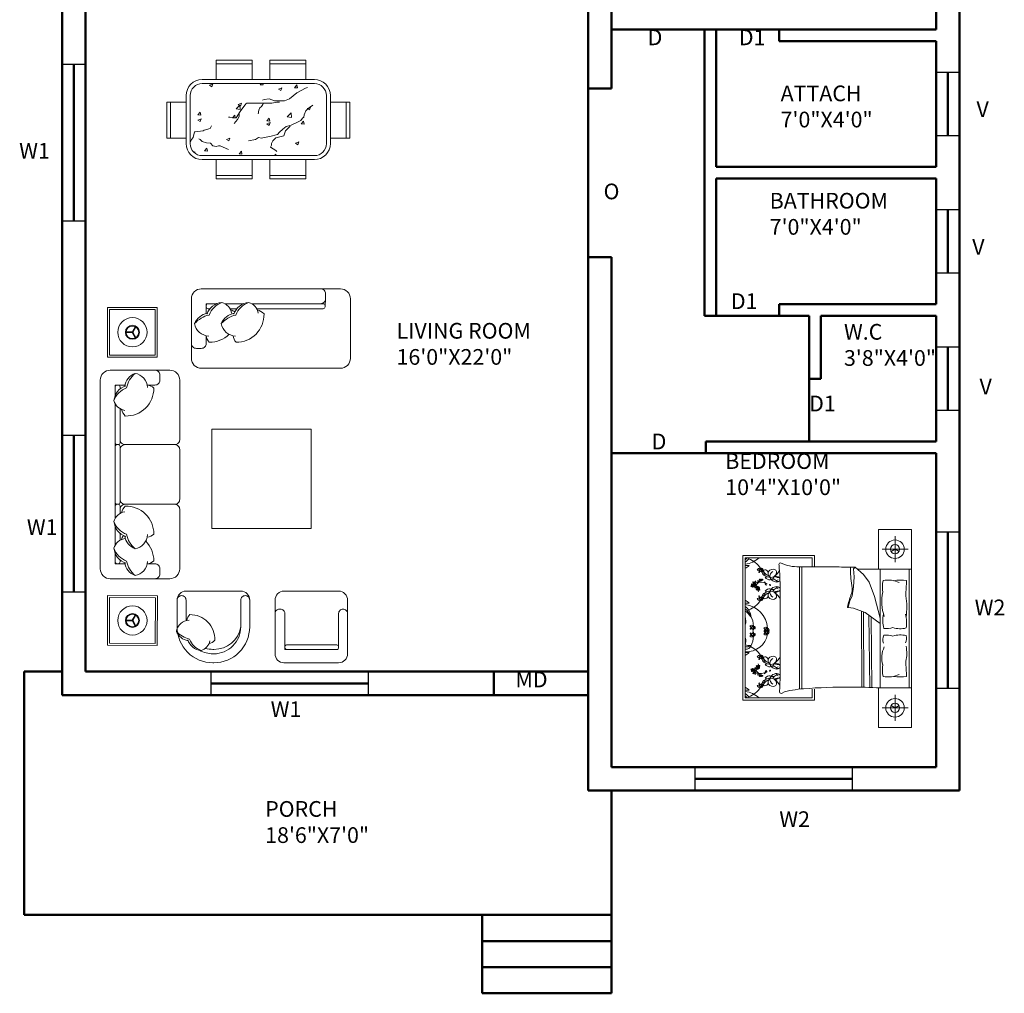
# Model space of a CAD drawing. Units: inches. Extents: x 18 to 447, y -515 to 49.
# Tile 1 of 2: x 71 to 447, y -515 to -143. Entities that reach past the tile are written whole.
import ezdxf

# ---------------------------------------------------------------- set-up
doc = ezdxf.new("R2010")
doc.units = ezdxf.units.IN
doc.header["$MEASUREMENT"] = 0
for name, color, linetype, lineweight in [('A-ANNO-TEXT', 7, 'Continuous', 25), ('A-AREA-IDEN', 3, 'Continuous', 25), ('A-FURN', 8, 'Continuous', 18), ('A-GLAZ', 4, 'Continuous', 25), ('A-WALL', 7, 'Continuous', 50)]:
    doc.layers.add(name, color=color, linetype=linetype, lineweight=lineweight)
doc.styles.get("Standard").update_dxf_attribs({"font": 'arial.ttf'})

# ---------------------------------------------------------------- blocks, each defined once
blk = doc.blocks.new('DAY BED1')
at = {"color": 0}
blk.add_line((0.3, 0.25), (0.225, 0.2549), dxfattribs=at)
blk.add_lwpolyline([(-0.3, 0, -0.414214), (-0.4, 0.1), (-0.4, 0.1, 0.317837), (-0.4, 0.1, -0.414214), (-0.4, 0.1), (-0.4, 0.1, 1.186185), (-0.4, 0.1, -0.414214), (-0.4, 0.1), (-0.4, 1.5, -0.414214), (-0.3, 1.6), (0.3, 1.6, -0.414214), (0.4, 1.5), (0.4, 0.1, -0.414214), (0.3, 0)], format="xyb", close=True, dxfattribs=at)
for points in [[(-0.0725, 1.45), (-0.15, 1.45, -0.414214), (-0.2, 1.5), (-0.2, 1.55, -0.414214), (-0.15, 1.6)], [(-0.0756, 1.4249, -0.356772), (0.0505, 1.5682, -0.249542), (0.1543, 1.4384, 9.61688)], [(0.0505, 1.5682, -0.14773), (0.1364, 1.422, -0.213343), (0.2624, 1.2931, -0.178662)], [(-0.0725, 1.4501, 0.165541), (-0.1386, 1.4192, 0.200231), (-0.0581, 1.2207, 0.121523)], [(0.1433, 1.4422, -0.306663), (0.2624, 1.2931, -0.30633), (0.1536, 1.1957, 0.872847)], [(0.25, 1.3448), (0.25, 1.45), (0.1517, 1.45, -0.414214)], [(0.2, 1.4118), (0.2, 1.43, -0.414214), (0.22, 1.45), (0.23, 1.45, -0.414214), (0.25, 1.43)], [(0.25, 1.43), (0.25, 1.3448, -0.414214)], [(-0.0756, 1.1556, -0.356772), (0.0505, 1.2988, -0.249542), (0.1543, 1.169, 9.61688)], [(0.0505, 1.2988, -0.14773), (0.1364, 1.1527, -0.213343), (0.2624, 1.0238, -0.178662)], [(0.1678, 1.1631, 0.071865), (0.1873, 1.205, -7.115464)], [(0.2, 1.1425), (0.2, 1.2113, -0.414214)], [(0.25, 1.2616), (0.25, 1.0755, -0.414214)], [(-0.0725, 1.1808, 0.165541), (-0.1386, 1.1498, 0.425989), (0.1479, 0.869, 0.121523), (0.1873, 0.9357, -7.115464)], [(0.1433, 1.1729, -0.306663), (0.2624, 1.0238, -0.30633), (0.1536, 0.9263, 0.872847)], [(0.25, 0.9923), (0.25, 0.2749, -0.414214), (0.23, 0.2549), (0.22, 0.2549, -0.414214), (0.2, 0.2749), (0.2, 0.9419, -0.414214)], [(0.25, 0.3775), (0.25, 0.3, 0.414214), (0.3, 0.25), (0.35, 0.25, 0.414214), (0.4, 0.3)]]:
    blk.add_lwpolyline(points, format="xyb", dxfattribs=at)
for points in [[(0.25, 1.0755), (0.25, 1.2616)], [(0.25, 0.3775), (0.25, 0.9923)]]:
    blk.add_lwpolyline(points, dxfattribs=at)
blk = doc.blocks.new('BED-DOUBLE')
for p, q in [((412.28, -42.96), (412.28, -33.06)), ((418.6, -30.43), (418.6, -106.23)), ((354.14, -40.44), (381.44, -40.44)), ((354.14, -95.69), (354.14, -40.44)), ((355.02, -41.31), (355.02, -94.82)), ((380.57, -41.31), (355.02, -41.31)), ((380.57, -44.72), (380.57, -41.31)), ((381.44, -40.44), (381.44, -44.72)), ((407.33, -38.01), (417.24, -38.01)), ((375.77, -91.48), (375.77, -44.72)), ((376.72, -91.41), (376.72, -44.72)), ((396.39, -45.53), (397.01, -44.91)), ((397.01, -44.91), (400.23, -47.67)), ((362.7, -48.78), (363.56, -48.62)), ((396.7, -48.6), (396.39, -45.53)), ((396.39, -52.43), (396.7, -48.6)), ((418.6, -45.59), (397.8, -45.59)), ((400.23, -47.67), (402.37, -50.59)), ((406.62, -45.59), (406.62, -91.07)), ((417.63, -91.07), (417.63, -45.59)), ((395.93, -55.81), (396.39, -52.43)), ((402.37, -50.59), (404.37, -56.12)), ((362.7, -54.08), (363.56, -54.25)), ((368.33, -83.72), (368.33, -52.94)), ((395.01, -57.81), (395.93, -55.81)), ((404.37, -56.12), (406.62, -64.38)), ((394.4, -60.26), (395.01, -57.81)), ((396.39, -60.57), (394.4, -60.26)), ((400.84, -62.26), (396.39, -60.57)), ((399.53, -90.8), (399.41, -61.72)), ((400.31, -90.8), (400.19, -62.01)), ((406.62, -66.41), (400.84, -62.26)), ((402.7, -90.83), (402.31, -63.31)), ((403.47, -90.86), (403.1, -63.88)), ((362.7, -82.05), (363.56, -81.88)), ((362.7, -87.35), (363.56, -87.51)), ((380.57, -94.82), (380.57, -91.47)), ((381.44, -91.49), (381.44, -95.69)), ((412.28, -93.7), (412.28, -103.6)), ((381.44, -95.69), (354.14, -95.69)), ((355.02, -94.82), (380.57, -94.82)), ((407.33, -98.65), (417.24, -98.65))]:
    blk.add_line(p, q)
for points in [[(405.97, -45.59), (405.97, -30.43), (418.6, -30.43)], [(412.28, -38.01), (410.75, -38.89)], [(412.28, -38.01), (413.82, -38.89)], [(418.6, -91.07), (405.97, -91.07), (405.97, -106.23), (418.6, -106.23)], [(412.28, -98.65), (410.75, -97.76)], [(412.28, -98.65), (413.82, -97.76)]]:
    blk.add_lwpolyline(points)
for points in [[(390.06, -44.75, 0.001242), (375.68, -44.72, -0.127202), (368.52, -43.2)], [(416.71, -49.94, 0.074897), (411.76, -50.04, -0.472817)], [(411.48, -67.97, 0.14099), (416.53, -68.13, 0.235245)], [(411.48, -71.21, -0.14099), (416.53, -71.06, -0.235245)], [(416.71, -86.71, -0.074897), (411.76, -86.62, 0.472817)], [(377.31, -91.39, 0.056112), (373.14, -91.94, 0.095341), (369.13, -93.01)]]:
    blk.add_lwpolyline(points, format="xyb")
for centre, radius in [((412.28, -38.01), 3.54), ((412.28, -38.01), 1.77), ((357.92, -51.9), 0.193), ((359.96, -53.16), 0.193), ((359.96, -82.97), 0.193), ((357.92, -84.23), 0.193), ((412.28, -98.65), 3.54), ((412.28, -98.65), 1.77)]:
    blk.add_circle(centre, radius)
for centre, radius, start, end in [((351.46, -37.17), 6.01, 306.3036, 316.4814), ((352.36, -38.91), 4.82, 303.4617, 330.1116), ((353.69, -33.94), 9.9, 277.745, 311.8856), ((353.48, -41.61), 4.02, 292.5547, 318.9546), ((355.64, -30.59), 13.69, 267.4081, 273.6519), ((352.71, -50.88), 9.9, 34.3865, 68.5908), ((368.56, -43.89), 0.699, 93.98, 207.3412), ((289.43, -52.04), 78.9, 359.3433, 5.6887), ((395.12, 24.59), 69.52, 265.8294, 271.553), ((423.85, -46.21), 28.61, 177.4519, 191.3392), ((360.64, -46.36), 1.1, 77.7115, 159.0387), ((360.05, -45.26), 0.827, 238.4633, 358.2869), ((362.76, -46.94), 2.5, 138.8402, 177.9352), ((360.38, -46.85), 0.123, 177.9352, 11.4834), ((360.44, -46.84), 0.0597, 11.4834, 127.9409), ((361.25, -46.01), 0.81, 117.6827, 223.7762), ((360.74, -46.49), 0.107, 223.7762, 159.7183), ((361.07, -46.09), 0.821, 2.9516, 103.728), ((367.63, -43.79), 6.92, 192.5173, 207.1824), ((359.96, -46.56), 1.56, 345.4653, 54.2343), ((362.32, -44.41), 1.69, 211.3827, 255.2969), ((362.98, -46.78), 1.42, 175.969, 254.3045), ((362.64, -47.05), 1.14, 350.264, 160.8688), ((361.41, -46.82), 0.697, 333.9755, 53.2681), ((361.1, -48.31), 1.51, 6.1662, 51.5825), ((365.15, -44.79), 3.58, 211.2614, 251.7045), ((364.86, -44.76), 4.07, 236.2883, 266.5076), ((364.34, -47.84), 1.88, 209.9085, 343.1337), ((365.56, -47.47), 1.81, 84.9449, 172.8857), ((365.96, -47.15), 2.2, 182.3591, 234.0401), ((366.25, -48.18), 1.76, 111.5819, 201.4221), ((364.8, -46.55), 2.28, 265.2933, 346.921), ((366.4, -51.29), 2.92, 122.7011, 126.3445), ((365.74, -46.94), 1.28, 354.4856, 91.0538), ((367.77, -45.7), 3.14, 238.8218, 279.1554), ((366.4, -51.29), 2.92, 55.785, 94.7304), ((362.99, -43.6), 5.74, 303.6671, 333.2997), ((367.49, -49.59), 0.913, 30.0293, 52.325), ((357.37, -52.19), 0.148, 142.4737, 265.053), ((357.56, -52.16), 0.319, 61.2196, 169.0403), ((357.4, -51.89), 0.449, 265.053, 338.3618), ((357.77, -51.51), 0.381, 157.4086, 261.4386), ((357.56, -51.49), 0.191, 58.0499, 135.6268), ((357.99, -52.51), 0.586, 113.4276, 137.6104), ((357.76, -51.61), 0.128, 172.906, 277.132), ((357.34, -51.85), 0.609, 14.7558, 58.0499), ((358.06, -52.25), 0.316, 139.7889, 227.6792), ((357.96, -52.36), 0.166, 227.6792, 350.3487), ((358.19, -51.69), 0.263, 36.1046, 181.4281), ((357.32, -52.24), 0.632, 353.0852, 15.7171), ((358.2, -50.65), 0.216, 124.3538, 214.3923), ((357.73, -52.32), 0.399, 350.3487, 43.6538), ((358.52, -50.69), 0.503, 190.3057, 287.1958), ((358.47, -51.91), 0.464, 198.7263, 262.5032), ((358.04, -51.48), 0.266, 270.0645, 331.1507), ((358.26, -51.54), 0.304, 221.8413, 265.7877), ((358.66, -50.51), 0.583, 176.9701, 248.2913), ((362.83, -47.43), 5.64, 212.6784, 216.3746), ((358.1, -52.12), 0.184, 1.1081, 91.8675), ((358.26, -51.66), 0.189, 263.7526, 41.7054), ((358.22, -52.17), 0.322, 11.5637, 86.365), ((358.47, -50.64), 0.223, 216.3746, 291.7548), ((360.44, -53.78), 3.15, 124.0033, 132.4917), ((358.45, -52.22), 0.149, 255.2356, 54.9248), ((357.21, -54.17), 3.36, 63.7819, 68.2913), ((359, -51.59), 0.535, 128.3208, 208.8162), ((359, -50.8), 0.503, 122.8155, 187.3992), ((359.1, -51.55), 0.639, 207.7043, 254.3516), ((358.61, -51.01), 0.168, 289.3605, 111.7548), ((358.74, -51.01), 0.168, 221.8703, 44.2646), ((359.5, -51.5), 0.88, 157.2305, 229.0635), ((359.22, -50.86), 0.583, 109.4799, 177.6828), ((359.21, -51.21), 0.518, 174.4544, 220.6188), ((358.68, -51.91), 0.88, 270.278, 342.111), ((359.27, -53.01), 0.622, 98.7227, 159.3375), ((356.26, -54.1), 3.78, 30.544, 49.818), ((358.91, -50.49), 0.216, 56.8636, 146.9021), ((359.02, -50.73), 0.223, 148.8844, 224.2646), ((358.34, -51.95), 0.622, 340.0041, 40.6188), ((363.66, -53.53), 5.64, 145.1882, 148.8844), ((360.44, -53.78), 3.15, 94.756, 119.2041), ((367.14, -58.31), 10.36, 132.2412, 142.1744), ((359.1, -51.89), 0.518, 278.7227, 324.8872), ((359, -52.31), 0.535, 290.5253, 358.5375), ((359.81, -52.77), 0.381, 157.4086, 261.4386), ((359.59, -52.76), 0.191, 58.0499, 135.6268), ((360.05, -52.15), 0.535, 182.8499, 266.1226), ((359.84, -51.78), 0.518, 231.7607, 277.9252), ((360.24, -51.68), 0.88, 214.5369, 286.3699), ((359.37, -53.11), 0.609, 14.7558, 58.0499), ((356.26, -54.1), 3.78, 23.0501, 23.8477), ((361.92, -50.06), 2.14, 178.3264, 187.1302), ((359.61, -50.36), 0.398, 11.3256, 64.4621), ((360.96, -49.79), 1.2, 190.2588, 210.656), ((360.15, -50.28), 0.364, 188.3432, 274.2869), ((360, -52.91), 0.622, 37.3105, 97.9252), ((360.47, -50.07), 0.635, 210.656, 242.6341), ((360.95, -49.53), 1.22, 218.2101, 226.3071), ((360.07, -52.05), 0.639, 265.0106, 311.658), ((360.05, -50.55), 0.154, 325.7657, 67.4417), ((355.26, -45.39), 7.2, 313.1541, 322.0459), ((360.6, -56.9), 6.28, 73.5842, 93.8277), ((360.55, -49.71), 0.148, 142.4737, 265.053), ((360.75, -49.68), 0.319, 127.7621, 169.0403), ((360.58, -49.41), 0.449, 265.053, 338.3618), ((361.17, -50.03), 0.586, 113.4276, 137.6104), ((361.1, -49.42), 0.193, 183.2768, 356.7232), ((361.25, -49.77), 0.316, 139.7889, 227.6792), ((361.15, -49.88), 0.166, 227.6792, 350.3487), ((360.5, -49.76), 0.632, 353.0852, 15.7171), ((360.92, -49.84), 0.399, 350.3487, 43.6538), ((361.66, -49.43), 0.464, 198.7263, 262.5032), ((361.29, -49.64), 0.184, 1.1081, 91.8675), ((361.63, -49.74), 0.149, 255.2356, 54.9248), ((361.4, -49.69), 0.322, 11.5637, 52.6358), ((364.47, -50.52), 2.14, 178.3264, 187.1302), ((362.16, -50.81), 0.398, 11.3256, 64.4621), ((363.51, -50.24), 1.2, 190.2588, 210.656), ((362.7, -50.73), 0.364, 188.3432, 274.2869), ((363.02, -50.53), 0.635, 210.656, 242.6341), ((363.5, -49.98), 1.22, 218.2101, 226.3071), ((362.6, -51), 0.154, 325.7657, 67.4417), ((363.04, -51.29), 0.364, 147.5332, 233.4768), ((363.37, -51.1), 0.635, 179.1859, 211.164), ((362.75, -51.24), 0.154, 354.3784, 96.0543), ((360.6, -56.9), 6.28, 63.0032, 69.8941), ((363.85, -50.81), 1.2, 211.164, 231.5612), ((364.06, -49.83), 2.14, 234.6898, 243.4936), ((364.07, -50.93), 1.22, 195.5129, 203.6099), ((362.71, -51.73), 0.398, 357.3579, 50.4944), ((364.42, -51.65), 0.146, 12.7051, 190.4384), ((364.51, -51.63), 0.238, 190.4384, 10.4136), ((365.13, -49.04), 0.47, 167.3041, 285.1471), ((366.95, -48.14), 2.42, 199.2822, 299.1751), ((366.95, -54.73), 2.42, 60.8249, 160.7178), ((365.66, -50.99), 1.55, 41.5653, 105.1471), ((366.51, -47.77), 2.18, 277.436, 299.9149), ((367.67, -49.21), 1.13, 221.5653, 293.8354), ((367.67, -53.66), 1.13, 66.1646, 138.4347), ((367.49, -49.59), 0.913, 314.4517, 333.558), ((367.49, -53.27), 0.913, 23.229, 45.5483), ((389.75, -53.05), 6.17, 336.2616, 11.3392), ((417.6, -52.65), 10.16, 165.1039, 191.0369), ((409.77, -59.6), 9.77, 65.1316, 101.7583), ((1138.04, -91.72), 722.54, 176.68521, 177.14978), ((358.96, -52.21), 0.639, 244.9899, 291.6373), ((359.4, -53.45), 0.148, 142.4737, 265.053), ((359.6, -53.42), 0.319, 61.2196, 169.0403), ((359.43, -53.16), 0.449, 265.053, 338.3618), ((360.02, -53.77), 0.586, 113.4276, 137.6104), ((359.79, -52.88), 0.128, 172.906, 277.132), ((360.1, -53.51), 0.316, 139.7889, 227.6792), ((360, -53.62), 0.166, 227.6792, 350.3487), ((360.23, -52.95), 0.263, 36.1046, 181.4281), ((359.35, -53.51), 0.632, 353.0852, 15.7171), ((356.26, -54.1), 3.78, 357.1071, 4.7585), ((359.77, -53.58), 0.399, 350.3487, 43.6538), ((360.07, -52.74), 0.266, 270.0645, 331.1507), ((360.3, -52.8), 0.304, 221.8413, 265.7877), ((360.51, -53.17), 0.464, 198.7263, 262.5032), ((360.14, -53.39), 0.184, 1.1081, 91.8675), ((360.38, -56.01), 0.123, 348.5166, 182.0648), ((362.76, -55.93), 2.5, 182.0648, 221.1598), ((360.3, -52.92), 0.189, 263.7526, 41.7054), ((360.26, -53.43), 0.322, 11.5637, 86.365), ((360.44, -56.03), 0.0597, 232.0591, 348.5166), ((361.25, -56.86), 0.81, 136.2238, 242.3173), ((360.49, -53.49), 0.149, 255.2356, 54.9248), ((360.78, -56.38), 0.0645, 200.2667, 136.2271), ((359.96, -56.3), 1.56, 305.7657, 14.5347), ((367.63, -59.08), 6.92, 152.8176, 167.4827), ((362.98, -56.09), 1.42, 105.6955, 184.031), ((362.64, -55.81), 1.14, 199.1312, 9.736), ((361.41, -56.05), 0.697, 306.7319, 26.0245), ((361.1, -54.56), 1.51, 308.4175, 353.8338), ((365.15, -58.07), 3.58, 108.2955, 148.7386), ((364.86, -58.1), 4.07, 93.4924, 123.7117), ((364.34, -55.02), 1.88, 16.8663, 150.0915), ((365.96, -55.71), 2.2, 125.9599, 177.6409), ((365.56, -55.4), 1.81, 187.1143, 275.0551), ((366.25, -54.69), 1.76, 158.5779, 248.4181), ((364.8, -56.31), 2.28, 13.079, 94.7067), ((365.13, -53.83), 0.47, 74.8529, 192.6959), ((366.4, -51.58), 2.92, 233.6555, 237.2989), ((365.66, -51.87), 1.55, 254.8529, 318.4347), ((365.74, -55.92), 1.28, 268.9462, 5.5144), ((367.77, -57.16), 3.14, 79.7133, 121.1782), ((366.4, -51.58), 2.92, 265.2696, 304.215), ((362.99, -59.26), 5.74, 21.4941, 56.3329), ((366.51, -55.09), 2.18, 60.0851, 82.564), ((367.49, -53.27), 0.913, 307.675, 336.7144), ((423.04, -65.53), 29.39, 160.1194, 169.3383), ((424.82, -57.99), 17.62, 168.0397, 199.2615), ((389.28, -60.33), 27.49, 352.2196, 9.497), ((353.48, -61.25), 4.02, 41.0454, 67.4453), ((355.64, -72.28), 13.69, 86.3481, 92.5919), ((353.69, -68.92), 9.9, 4.4623, 82.255), ((352.36, -63.95), 4.82, 1.272, 56.5383), ((352.71, -51.98), 9.9, 291.4092, 325.6135), ((360.05, -57.6), 0.827, 1.7131, 121.5367), ((360.64, -56.5), 1.1, 200.9613, 282.2885), ((361.07, -56.78), 0.821, 256.272, 357.0484), ((362.32, -58.45), 1.69, 104.7031, 148.6173), ((394.34, -60.09), 0.183, 178.8623, 289.7536), ((351.46, -65.69), 6.01, 17.8504, 53.6964), ((349.77, -68.85), 8.94, 34.0123, 54.053), ((349.81, -65.39), 5.44, 343.5431, 17.0202), ((348.38, -68.16), 9.9, 4.4623, 27.4146), ((420.97, -65.13), 13.37, 169.8617, 193.6238), ((403.18, -66.14), 13.51, 351.5249, 13.96), ((347.01, -67.55), 8.05, 4.3787, 5.6357), ((341.5, -71.79), 14.38, 19.7217, 19.9028), ((357.51, -68.2), 1.1, 47.7873, 129.1145), ((357.55, -66.96), 0.827, 208.5391, 328.3627), ((359.06, -69.76), 2.5, 108.9159, 148.011), ((358.22, -68.2), 0.81, 87.7585, 193.852), ((364.86, -69.46), 6.92, 162.593, 177.2582), ((356.83, -68.03), 1.56, 315.5411, 24.3101), ((359.94, -67.35), 1.69, 181.4585, 225.3727), ((358.02, -68.18), 0.821, 333.0274, 73.8037), ((355.97, -69.42), 7.66, 262.8636, 351.8197), ((357.55, -71.7), 0.827, 31.6373, 151.4609), ((357.51, -70.45), 1.1, 230.8855, 312.2127), ((357.04, -68.5), 0.123, 148.011, 341.5592), ((357.04, -70.16), 0.123, 18.4408, 211.989), ((359.06, -68.9), 2.5, 211.989, 251.0841), ((357.1, -68.52), 0.0597, 341.5592, 98.0167), ((357.1, -70.14), 0.0597, 261.9833, 18.4408), ((348.38, -70.5), 9.9, 332.5854, 355.5377), ((358.22, -70.46), 0.81, 166.148, 272.2415), ((357.54, -68.37), 0.107, 193.852, 129.9245), ((357.58, -70.28), 0.0645, 230.1909, 166.0209), ((364.86, -69.19), 6.92, 182.7418, 197.407), ((356.83, -70.62), 1.56, 335.6899, 44.4589), ((359.94, -71.31), 1.69, 134.6273, 178.5415), ((358.02, -70.48), 0.821, 286.1963, 26.9726), ((362.82, -68.96), 1.1, 47.7873, 129.1145), ((362.85, -67.71), 0.827, 208.5391, 328.3627), ((362.85, -70.94), 0.827, 31.6373, 151.4609), ((362.82, -69.69), 1.1, 230.8855, 312.2127), ((362.35, -69.26), 0.123, 148.011, 341.5592), ((362.35, -69.4), 0.123, 18.4408, 211.989), ((364.36, -70.52), 2.5, 108.9159, 148.011), ((364.36, -68.14), 2.5, 211.989, 251.0841), ((362.41, -69.28), 0.0597, 341.5592, 98.0167), ((362.41, -69.38), 0.0597, 261.9833, 18.4408), ((363.52, -68.96), 0.81, 87.7585, 193.852), ((363.52, -69.7), 0.81, 166.148, 272.2415), ((362.84, -69.13), 0.107, 193.852, 129.9245), ((362.88, -69.52), 0.0645, 230.1909, 166.0209), ((362.13, -68.79), 1.56, 315.5411, 24.3101), ((370.16, -70.22), 6.92, 162.593, 177.2582), ((362.13, -69.86), 1.56, 335.6899, 44.4589), ((370.16, -68.44), 6.92, 182.7418, 197.407), ((363.32, -68.94), 0.821, 333.0274, 73.8037), ((365.24, -68.11), 1.69, 181.4585, 225.3727), ((363.32, -69.72), 0.821, 286.1963, 26.9726), ((365.24, -70.55), 1.69, 134.6273, 178.5415), ((411.62, -72.61), 4.02, 155.0183, 198.5407), ((408.95, -59.04), 9.29, 264.0129, 285.8293), ((408.95, -80.15), 9.29, 74.1707, 95.9871), ((412.93, -72.1), 3.75, 333.3437, 16.1026), ((349.81, -73.26), 5.44, 342.9798, 16.4569), ((347.01, -71.11), 8.05, 354.3643, 355.6213), ((341.5, -66.87), 14.38, 340.0972, 340.2783), ((356.67, -70.41), 4.43, 248.117, 276.6195), ((355.44, -74.47), 1.78, 256.3898, 349.0739), ((355.68, -73.14), 2.25, 252.8609, 311.9049), ((352.71, -84.14), 9.9, 34.3865, 68.5908), ((403.45, -77.72), 13.32, 346.3427, 11.1841), ((355.64, -63.85), 13.69, 267.4081, 273.6519), ((353.48, -74.88), 4.02, 292.5547, 318.9546), ((360.64, -79.63), 1.1, 77.7115, 159.0387), ((360.05, -78.53), 0.827, 238.4633, 358.2869), ((362.76, -80.2), 2.5, 138.8402, 177.9352), ((361.25, -79.27), 0.81, 117.6827, 223.7762), ((361.07, -79.35), 0.821, 2.9516, 103.728), ((362.32, -77.67), 1.69, 211.3827, 255.2969), ((359.96, -79.82), 1.56, 345.4653, 54.2343), ((367.63, -77.05), 6.92, 192.5173, 207.1824), ((365.56, -80.73), 1.81, 84.9449, 172.8857), ((365.74, -80.21), 1.28, 354.4856, 91.0538), ((362.99, -76.87), 5.74, 303.6671, 338.5059), ((416.85, -79.63), 9.65, 153.8761, 196.1746), ((359.4, -82.67), 0.148, 94.947, 217.5263), ((359.6, -82.7), 0.319, 190.9597, 298.7804), ((359.43, -82.97), 0.449, 21.6382, 94.947), ((360.02, -82.36), 0.586, 222.3896, 246.5724), ((360.1, -82.62), 0.316, 132.3208, 220.2111), ((360, -82.51), 0.166, 9.6513, 132.3208), ((359.35, -82.62), 0.632, 344.2829, 6.9148), ((356.26, -82.03), 3.78, 355.2415, 2.8929), ((359.77, -82.55), 0.399, 316.3462, 9.6513), ((360.51, -82.96), 0.464, 97.4968, 161.2737), ((360.14, -82.74), 0.184, 268.1325, 358.8919), ((360.38, -80.12), 0.123, 177.9352, 11.4834), ((360.26, -82.7), 0.322, 273.635, 348.4363), ((360.44, -80.1), 0.0597, 11.4834, 127.9409), ((360.49, -82.64), 0.149, 305.0752, 104.7644), ((360.74, -79.76), 0.107, 223.7762, 159.7183), ((362.98, -80.04), 1.42, 175.969, 254.3045), ((362.64, -80.32), 1.14, 350.264, 160.8688), ((361.41, -80.08), 0.697, 333.9755, 53.2681), ((361.1, -81.57), 1.51, 6.1662, 51.5825), ((365.15, -78.06), 3.58, 211.2614, 251.7045), ((364.86, -78.03), 4.07, 236.2883, 266.5076), ((364.34, -81.11), 1.88, 209.9085, 343.1337), ((365.96, -80.42), 2.2, 182.3591, 234.0401), ((366.25, -81.44), 1.76, 111.5819, 201.4221), ((364.8, -79.81), 2.28, 265.2933, 346.921), ((365.13, -82.3), 0.47, 167.3041, 285.1471), ((366.4, -84.55), 2.92, 122.7011, 126.3445), ((366.95, -81.4), 2.42, 199.2822, 299.1751), ((365.66, -84.26), 1.55, 41.5653, 105.1471), ((367.77, -78.97), 3.14, 238.8218, 280.2867), ((366.4, -84.55), 2.92, 55.785, 94.7304), ((367.49, -82.86), 0.913, 23.2856, 52.325), ((417.6, -84.01), 10.16, 168.9631, 194.8961), ((1138.04, -44.94), 722.54, 182.85022, 183.31479), ((357.37, -83.94), 0.148, 94.947, 217.5263), ((357.56, -83.97), 0.319, 190.9597, 298.7804), ((357.4, -84.24), 0.449, 21.6382, 94.947), ((357.77, -84.62), 0.381, 98.5614, 202.5914), ((357.56, -84.64), 0.191, 224.3732, 301.9501), ((357.99, -83.62), 0.586, 222.3896, 246.5724), ((357.76, -84.52), 0.128, 82.868, 187.094), ((357.34, -84.28), 0.609, 301.9501, 345.2442), ((358.06, -83.88), 0.316, 132.3208, 220.2111), ((357.96, -83.77), 0.166, 9.6513, 132.3208), ((357.32, -83.88), 0.632, 344.2829, 6.9148), ((358.19, -84.44), 0.263, 178.5719, 323.8954), ((358.2, -85.47), 0.216, 145.6077, 235.6462), ((357.73, -83.81), 0.399, 316.3462, 9.6513), ((358.47, -84.22), 0.464, 97.4968, 161.2737), ((358.52, -85.44), 0.503, 72.8042, 169.6943), ((358.26, -84.59), 0.304, 94.2123, 138.1587), ((358.04, -84.65), 0.266, 28.8493, 89.9355), ((358.66, -85.62), 0.583, 111.7087, 183.0299), ((362.83, -88.7), 5.64, 143.6254, 147.3216), ((358.1, -84), 0.184, 268.1325, 358.8919), ((358.22, -83.96), 0.322, 273.635, 348.4363), ((358.26, -84.47), 0.189, 318.2946, 96.2474), ((358.47, -85.49), 0.223, 68.2452, 143.6254), ((360.44, -82.35), 3.15, 227.5083, 235.9967), ((358.45, -83.91), 0.149, 305.0752, 104.7644), ((357.21, -81.96), 3.36, 291.7087, 296.2181), ((359, -84.54), 0.535, 151.1838, 231.6792), ((359, -85.33), 0.503, 172.6008, 237.1845), ((359.1, -84.58), 0.639, 105.6484, 152.2957), ((358.61, -85.12), 0.168, 248.2452, 70.6395), ((358.74, -85.12), 0.168, 315.7354, 138.1297), ((359.5, -84.63), 0.88, 130.9365, 202.7695), ((359.22, -85.26), 0.583, 182.3172, 250.5201), ((358.96, -83.92), 0.639, 68.3627, 115.0101), ((358.68, -84.22), 0.88, 17.889, 89.722), ((359.27, -83.12), 0.622, 200.6625, 261.2773), ((359.21, -84.92), 0.518, 139.3812, 185.5456), ((356.26, -82.03), 3.78, 310.182, 329.456), ((358.91, -85.63), 0.216, 213.0979, 303.1364), ((359.02, -85.39), 0.223, 135.7354, 211.1156), ((358.34, -84.18), 0.622, 319.3812, 19.9959), ((363.66, -82.6), 5.64, 211.1156, 214.8118), ((360.44, -82.35), 3.15, 240.7959, 265.244), ((367.14, -77.82), 10.36, 217.8256, 227.7588), ((359.1, -84.24), 0.518, 35.1128, 81.2773), ((359, -83.82), 0.535, 1.4625, 69.4747), ((359.81, -83.36), 0.381, 98.5614, 202.5914), ((359.59, -83.37), 0.191, 224.3732, 301.9501), ((360.05, -83.98), 0.535, 93.8774, 177.1501), ((360.24, -84.44), 0.88, 73.6301, 145.4631), ((359.84, -84.35), 0.518, 82.0748, 128.2393), ((359.79, -83.25), 0.128, 82.868, 187.094), ((359.37, -83.02), 0.609, 301.9501, 345.2442), ((356.26, -82.03), 3.78, 336.1523, 336.9499), ((360.96, -86.34), 1.2, 149.344, 169.7412), ((361.92, -86.07), 2.14, 172.8698, 181.6736), ((359.61, -85.77), 0.398, 295.5379, 348.6744), ((360.15, -85.85), 0.364, 85.7131, 171.6568), ((360, -83.22), 0.622, 262.0748, 322.6895), ((360.47, -86.05), 0.635, 117.3659, 149.344), ((360.23, -83.18), 0.263, 178.5719, 323.8954), ((360.95, -86.6), 1.22, 133.6929, 141.7899), ((360.07, -84.08), 0.639, 48.342, 94.9894), ((360.3, -83.32), 0.304, 94.2123, 138.1587), ((360.07, -83.39), 0.266, 28.8493, 89.9355), ((360.05, -85.58), 0.154, 292.5583, 34.2343), ((360.6, -79.23), 6.28, 266.1723, 286.4158), ((355.26, -90.74), 7.2, 37.9541, 46.8459), ((360.3, -83.21), 0.189, 318.2946, 96.2474), ((360.55, -86.42), 0.148, 94.947, 217.5263), ((360.75, -86.45), 0.319, 190.9597, 232.2379), ((360.58, -86.72), 0.449, 21.6382, 94.947), ((361.17, -86.1), 0.586, 222.3896, 246.5724), ((361.1, -86.71), 0.193, 3.2768, 176.7232), ((361.25, -86.36), 0.316, 132.3208, 220.2111), ((361.15, -86.25), 0.166, 9.6513, 132.3208), ((360.5, -86.36), 0.632, 344.2829, 6.9148), ((360.92, -86.29), 0.399, 316.3462, 9.6513), ((361.66, -86.7), 0.464, 97.4968, 161.2737), ((361.29, -86.48), 0.184, 268.1325, 358.8919), ((361.63, -86.38), 0.149, 305.0752, 104.7644), ((361.4, -86.44), 0.322, 307.3642, 348.4363), ((363.51, -85.89), 1.2, 149.344, 169.7412), ((364.47, -85.61), 2.14, 172.8698, 181.6736), ((362.16, -85.32), 0.398, 295.5379, 348.6744), ((362.7, -85.4), 0.364, 85.7131, 171.6568), ((363.02, -85.6), 0.635, 117.3659, 149.344), ((363.5, -86.15), 1.22, 133.6929, 141.7899), ((362.6, -85.13), 0.154, 292.5583, 34.2343), ((363.04, -84.84), 0.364, 126.5232, 212.4668), ((364.34, -88.29), 1.88, 16.8663, 150.0915), ((363.37, -85.03), 0.635, 148.836, 180.8141), ((362.75, -84.88), 0.154, 263.9457, 5.6216), ((360.6, -79.23), 6.28, 290.1059, 296.9968), ((363.85, -85.32), 1.2, 128.4388, 148.836), ((364.06, -86.3), 2.14, 116.5064, 125.3102), ((364.07, -85.2), 1.22, 156.3901, 164.4871), ((362.71, -84.4), 0.398, 309.5056, 2.6421), ((364.51, -84.5), 0.238, 349.5864, 169.5616), ((364.42, -84.48), 0.146, 169.5616, 347.2949), ((366.95, -87.99), 2.42, 60.8249, 160.7178), ((365.66, -85.14), 1.55, 254.8529, 318.4347), ((366.51, -81.04), 2.18, 277.436, 299.9149), ((366.51, -88.36), 2.18, 60.0851, 82.564), ((367.67, -82.47), 1.13, 221.5653, 293.8354), ((367.67, -86.92), 1.13, 66.1646, 138.4347), ((294.61, -86.04), 73.76, 355.2402, 1.8035), ((367.49, -82.86), 0.913, 314.4517, 336.7144), ((367.49, -86.54), 0.913, 16.6343, 45.5483), ((409.77, -77.06), 9.77, 258.2417, 294.8684), ((360.05, -90.87), 0.827, 1.7131, 121.5367), ((360.64, -89.77), 1.1, 200.9613, 282.2885), ((360.38, -89.28), 0.123, 348.5166, 182.0648), ((362.76, -89.19), 2.5, 182.0648, 221.1598), ((360.44, -89.29), 0.0597, 232.0591, 348.5166), ((361.25, -90.12), 0.81, 136.2238, 242.3173), ((360.78, -89.65), 0.0645, 200.2667, 136.2271), ((367.63, -92.34), 6.92, 152.8176, 167.4827), ((359.96, -89.57), 1.56, 305.7657, 14.5347), ((362.32, -91.72), 1.69, 104.7031, 148.6173), ((361.07, -90.04), 0.821, 256.272, 357.0484), ((362.98, -89.35), 1.42, 105.6955, 184.031), ((362.64, -89.08), 1.14, 199.1312, 9.736), ((361.41, -89.31), 0.697, 306.7319, 26.0245), ((361.1, -87.82), 1.51, 308.4175, 353.8338), ((365.15, -91.34), 3.58, 108.2955, 148.7386), ((364.86, -91.37), 4.07, 93.4924, 123.7117), ((365.96, -88.98), 2.2, 125.9599, 177.6409), ((365.56, -88.66), 1.81, 187.1143, 275.0551), ((366.25, -87.95), 1.76, 158.5779, 248.4181), ((364.8, -89.58), 2.28, 13.079, 94.7067), ((365.13, -87.09), 0.47, 74.8529, 192.6959), ((366.4, -84.84), 2.92, 233.6555, 237.2989), ((365.74, -89.19), 1.28, 268.9462, 5.5144), ((367.77, -90.43), 3.14, 79.249, 121.1782), ((366.4, -84.84), 2.92, 265.2696, 304.215), ((362.99, -92.53), 5.74, 23.6453, 56.3329), ((367.49, -86.54), 0.913, 307.675, 342.5814), ((353.48, -94.52), 4.02, 41.0454, 67.4453), ((355.64, -105.54), 13.69, 86.3481, 92.5919), ((353.69, -102.18), 9.9, 48.1144, 82.255), ((352.36, -97.22), 4.82, 29.8884, 56.5383), ((352.71, -85.25), 9.9, 291.4092, 325.6135), ((368.74, -92.43), 0.691, 156.5219, 303.8264), ((392.41, -268.41), 177.66, 89.1145, 94.8735), ((397.36, -226.95), 136.19, 86.1, 90.9282), ((351.46, -98.95), 6.01, 43.5186, 53.6964)]:
    blk.add_arc(centre, radius, start, end)
blk = doc.blocks.new('SIDE-TABLE-LAMP')
for p, q in [((114.05, -262.6), (111.38, -262.6)), ((114.05, -262.84), (111.38, -262.84)), ((113.95, -262.66), (115.29, -260.34)), ((113.95, -262.78), (115.29, -265.1)), ((114.16, -262.78), (115.5, -260.46)), ((114.16, -262.66), (115.5, -264.98))]:
    blk.add_line(p, q)
at = {"ltscale": 0.03}
blk.add_lwpolyline([(123.55, -253.23), (123.55, -272.22), (104.56, -272.22), (104.56, -253.23)], close=True, dxfattribs=at)
blk.add_lwpolyline([(122.79, -271.46), (122.79, -253.99), (105.32, -253.99), (105.32, -271.46)], close=True)
for radius in [5.6, 2.68, 2.4]:
    blk.add_circle((114.05, -262.72), radius)
blk = doc.blocks.new('CHAIR-DINING')
for p, q in [((7.38, 13.77), (0, 13.77)), ((7.38, 0), (7.38, 13.77)), ((0, 0), (7.38, 0))]:
    blk.add_line(p, q)
blk = doc.blocks.new('WIN-W')
for p, q in [((0, 9), (60, 9)), ((0, 0), (0, 9)), ((60, 9), (60, 0)), ((60, 0), (0, 0))]:
    blk.add_line(p, q)
blk = doc.blocks.new('WIN-V')
for p, q in [((0, 24), (0, 0)), ((9, 24), (0, 24)), ((9, 0), (9, 24)), ((0, 0), (9, 0))]:
    blk.add_line(p, q)

msp = doc.modelspace()

# ---------------------------------------------------------------- linework, layer by layer
at = {"layer": 'A-FURN'}
for p, q in [((159.8, -160.07), (146.02, -160.07)), ((180.31, -160.07), (166.53, -160.07)), ((183.58, -166.1), (140.73, -166.1)), ((140.73, -167.63), (183.58, -167.63)), ((143.51, -168.24), (144.8, -167.75)), ((143.51, -168.24), (144.42, -168.86)), ((144.42, -168.86), (144.8, -167.75)), ((162.87, -168.05), (163.22, -167.63)), ((162.87, -168.05), (163.97, -168.15)), ((163.97, -168.15), (163.87, -167.63)), ((169.9, -169.71), (171.19, -169.22)), ((170.82, -170.33), (171.19, -169.22)), ((176.04, -169.2), (176.93, -168.15)), ((176.04, -169.2), (177.14, -169.3)), ((177.14, -169.3), (176.93, -168.15)), ((181.02, -169.11), (180.19, -169.44)), ((134.61, -172.22), (134.61, -190.59)), ((136.14, -190.59), (136.14, -172.22)), ((169.9, -169.71), (170.82, -170.33)), ((176.86, -171.11), (174.03, -173.43)), ((180.19, -169.44), (176.86, -171.11)), ((188.17, -172.22), (188.17, -190.59)), ((189.7, -190.59), (189.7, -172.22)), ((128.58, -188.48), (128.58, -174.7)), ((153.65, -177.31), (155.08, -175.82)), ((154.47, -175.64), (155.76, -175.14)), ((154.47, -175.64), (155.39, -176.25)), ((155.28, -177.56), (155.08, -175.82)), ((157.39, -175.43), (155.22, -178.25)), ((155.39, -176.25), (155.76, -175.14)), ((157.72, -175.1), (157.39, -175.43)), ((167.37, -175.1), (157.72, -175.1)), ((163.38, -176.42), (162.72, -176.92)), ((163.88, -175.59), (163.38, -176.42)), ((164.38, -173.77), (163.71, -173.93)), ((164.21, -175.09), (163.88, -175.59)), ((166.37, -173.43), (164.38, -173.77)), ((168.37, -174.26), (166.37, -173.43)), ((169.2, -174.76), (167.37, -175.1)), ((172.2, -174.26), (168.37, -174.26)), ((170.2, -174.76), (169.2, -174.76)), ((174.03, -173.43), (172.2, -174.26)), ((181.68, -176.76), (180.35, -178.09)), ((180.86, -177.11), (182.15, -176.61)), ((183.02, -175.93), (181.68, -176.76)), ((181.78, -177.72), (182.15, -176.61)), ((195.73, -174.7), (195.73, -188.48)), ((139.07, -179.56), (139.96, -178.51)), ((139.07, -179.56), (140.17, -179.66)), ((140.17, -179.66), (139.96, -178.51)), ((151.23, -180.42), (150.73, -180.42)), ((153.73, -180.75), (151.23, -180.42)), ((152.24, -180.71), (153.13, -179.66)), ((153.34, -180.81), (153.13, -179.66)), ((153.65, -177.31), (155.28, -177.56)), ((155.22, -178.25), (153.73, -180.75)), ((154.89, -180.25), (154.23, -181.41)), ((154.89, -178.75), (154.89, -180.25)), ((162.22, -178.75), (162.05, -179.25)), ((162.38, -177.75), (162.22, -178.41)), ((162.22, -178.41), (162.22, -178.75)), ((162.72, -176.92), (162.38, -177.75)), ((173.25, -180.35), (174.68, -178.85)), ((173.25, -180.35), (174.88, -180.6)), ((174.88, -180.6), (174.68, -178.86)), ((179.52, -180.42), (179.02, -180.91)), ((179.69, -179.58), (179.52, -180.42)), ((180.35, -178.09), (179.69, -179.58)), ((180.86, -177.11), (181.78, -177.72)), ((139.04, -181.56), (140.33, -181.07)), ((139.04, -181.56), (139.95, -182.18)), ((139.95, -182.18), (140.33, -181.07)), ((143.74, -184.74), (144.24, -183.74)), ((152.24, -180.71), (153.34, -180.81)), ((153.56, -182.08), (152.89, -182.91)), ((154.23, -181.41), (153.56, -182.08)), ((165.42, -181.87), (166.3, -180.81)), ((165.42, -181.87), (166.51, -181.96)), ((165.43, -183.03), (166.72, -182.54)), ((165.43, -183.03), (166.35, -183.65)), ((166.51, -181.96), (166.3, -180.81)), ((166.35, -183.65), (166.72, -182.54)), ((172.86, -184.07), (171.53, -185.07)), ((174.69, -183.57), (172.86, -184.07)), ((174.36, -183.91), (173.7, -184.57)), ((177.19, -182.41), (174.69, -183.57)), ((178.36, -181.74), (177.19, -182.41)), ((179.02, -180.91), (178.36, -181.74)), ((178.59, -183.02), (179.47, -181.96)), ((178.59, -183.02), (179.69, -183.11)), ((179.69, -183.12), (179.47, -181.96)), ((137.25, -188.23), (137.75, -186.07)), ((137.75, -186.07), (138.08, -186.07)), ((138.08, -186.07), (141.08, -185.73)), ((141.08, -185.73), (141.41, -185.4)), ((141.41, -185.4), (143.74, -184.74)), ((166.54, -187.89), (164.38, -188.23)), ((169.54, -187.06), (166.54, -187.89)), ((171.87, -187.56), (168.87, -188.39)), ((170.2, -186.23), (169.54, -187.06)), ((171.53, -185.07), (170.2, -186.23)), ((172.03, -187.23), (171.87, -187.56)), ((172.53, -185.73), (172.03, -187.23)), ((173.7, -184.57), (172.53, -185.73)), ((136.25, -189.89), (136.59, -189.06)), ((136.59, -189.06), (137.25, -188.23)), ((139.92, -189.05), (139.42, -188.72)), ((140.75, -189.72), (139.92, -189.05)), ((142.41, -190.22), (140.75, -189.72)), ((143.91, -190.38), (142.41, -190.22)), ((144.74, -191.38), (143.91, -190.38)), ((146.07, -191.71), (144.74, -191.38)), ((146.91, -191.38), (146.07, -191.71)), ((147.57, -191.38), (146.91, -191.38)), ((150.73, -192.88), (147.57, -191.38)), ((150, -188.95), (151.29, -188.46)), ((150, -188.95), (150.92, -189.57)), ((150.92, -189.57), (151.29, -188.46)), ((161.05, -189.06), (158.39, -189.56)), ((162.21, -188.23), (161.05, -189.06)), ((163.38, -188.56), (162.21, -188.23)), ((164.38, -188.23), (163.38, -188.56)), ((167.21, -191.22), (166.87, -191.88)), ((166.87, -191.88), (168.87, -193.21)), ((167.71, -189.56), (167.21, -190.55)), ((167.21, -190.55), (167.21, -191.22)), ((168.87, -188.39), (167.71, -189.56)), ((176.4, -190.43), (177.68, -189.93)), ((176.4, -190.43), (177.31, -191.04)), ((177.31, -191.04), (177.68, -189.93)), ((137.64, -193.99), (137.91, -193.71)), ((137.98, -194.26), (137.91, -193.71)), ((183.58, -195.18), (140.73, -195.18)), ((141.62, -193.38), (142.5, -192.32)), ((141.62, -193.38), (142.72, -193.47)), ((142.72, -193.47), (142.5, -192.32)), ((154.79, -194.53), (155.68, -193.47)), ((154.79, -194.53), (155.89, -194.62)), ((155.89, -194.62), (155.68, -193.47)), ((168.39, -195.18), (168.85, -194.63)), ((168.95, -195.18), (168.85, -194.63)), ((168.87, -193.21), (169.2, -193.55)), ((140.73, -196.71), (183.58, -196.71)), ((159.8, -202.74), (146.02, -202.74)), ((180.31, -202.74), (166.53, -202.74))]:
    msp.add_line(p, q, dxfattribs=at)
at = {"layer": 'A-FURN', "ltscale": 0.03}
for points in [[(128.35, -277.2, -0.414214), (132.14, -281), (132.14, -303.79, -0.414214), (130.24, -305.68, -0.414214), (132.14, -307.58), (132.14, -326.57, -0.414214), (130.24, -328.47, -0.414214), (132.14, -330.37), (132.14, -353.15, -0.414214), (128.35, -356.95), (105.56, -356.95, -0.414214), (101.76, -353.15), (101.76, -281, -0.414214), (105.56, -277.2)], [(192.86, -389.08), (192.86, -389.08, 0.414214), (196.28, -385.65), (196.28, -365.11, 0.414214), (192.86, -361.69), (192.86, -361.69), (171.97, -361.69, 0.414214), (168.55, -365.11), (168.55, -385.65, 0.414214), (171.97, -389.08)]]:
    msp.add_lwpolyline(points, format="xyb", close=True, dxfattribs=at)
at = {"layer": 'A-FURN'}
for points in [[(115.04, -278.41, 0.14773), (111.77, -283.96, 0.213343), (106.99, -288.86, 0.178662)], [(119.82, -283.85, 0.356772), (115.04, -278.41, 0.249542), (111.09, -283.34, -9.61688)], [(122.65, -277.2, -0.414214), (124.55, -279.1), (124.55, -281, -0.414214), (122.65, -282.9), (119.71, -282.9)], [(111.51, -283.19, 0.306663), (106.99, -288.86, 0.30633), (111.12, -292.56, -0.872847)], [(109.36, -284.35), (109.36, -283.66, 0.414214), (108.6, -282.9), (108.22, -282.9, 0.414214), (107.46, -283.66)], [(107.46, -283.66), (107.46, -286.89, 0.414214)], [(119.71, -282.9, -0.165541), (122.22, -284.07, -0.425989), (111.34, -294.73, -0.121523), (109.84, -292.2, 7.115464)], [(107.46, -290.05), (107.46, -304.93, 0.414214), (108.22, -305.68), (108.6, -305.68, 0.414214), (109.36, -304.93), (109.36, -291.96, 0.414214)], [(109.36, -303.79, 0.414214), (111.26, -305.68), (130.24, -305.68, 0.414214)], [(109.36, -307.58, -0.414214), (111.26, -305.68)], [(109.36, -326.57, 0.414214), (111.26, -328.47)], [(107.46, -333.87), (107.46, -329.23, -0.414214), (108.22, -328.47), (108.6, -328.47, -0.414214), (109.36, -329.23), (109.36, -331.96, -0.414214)], [(109.36, -330.37, -0.414214), (111.26, -328.47), (130.24, -328.47, -0.414214)], [(119.71, -341.03, 0.165541), (122.22, -339.86, 0.425989), (111.34, -329.19, 0.121523), (109.84, -331.72, -7.115464)], [(111.51, -340.73, -0.306663), (106.99, -335.07, -0.30633), (111.12, -331.37, 0.872847)], [(115.04, -345.51, -0.14773), (111.77, -339.96, -0.213343), (106.99, -335.07, -0.178662)], [(107.46, -344.1), (107.46, -337.03, -0.414214)], [(111.51, -350.96, -0.306663), (106.99, -345.3, -0.30633), (111.12, -341.6, 0.872847)], [(109.36, -339.58), (109.36, -342.19, -0.414214)], [(110.58, -340.36, 0.071865), (109.84, -341.95, -7.115464)], [(119.82, -340.07, -0.356772), (115.04, -345.51, -0.249542), (111.09, -340.58, 9.61688)], [(115.04, -355.74, -0.14773), (111.77, -350.19, -0.213343), (106.99, -345.3, -0.178662)], [(119.71, -351.26, 0.165541), (122.22, -350.08, 0.200231), (119.16, -342.55, 0.121523)], [(107.46, -347.26), (107.46, -351.25), (111.19, -351.25, -0.414214)], [(107.46, -350.5), (107.46, -347.26, -0.414214)], [(109.36, -349.81), (109.36, -350.5, -0.414214), (108.6, -351.25), (108.22, -351.25, -0.414214), (107.46, -350.5)], [(119.82, -350.3, -0.356772), (115.04, -355.74, -0.249542), (111.09, -350.81, 9.61688)], [(119.71, -351.25), (122.65, -351.25, -0.414214), (124.55, -353.15), (124.55, -355.05, -0.414214), (122.65, -356.95)], [(134.56, -372.98), (134.56, -365.11, 0.414214), (132.85, -363.4), (132.85, -363.4, 0.414214), (131.14, -365.11)], [(155.45, -375.38), (155.45, -365.11, -0.414214), (157.16, -363.4), (157.16, -363.4, -0.414214), (158.87, -365.11)], [(168.55, -370.25, -0.414214), (170.26, -368.53), (170.6, -368.53, -0.414214), (172.32, -370.25), (172.32, -372.9)], [(192.86, -382.92), (192.86, -370.25, -0.414214), (194.57, -368.53), (194.57, -368.53, -0.414214), (196.28, -370.25)], [(134.9, -372.9, -0.165541), (135.96, -370.64, -0.425989), (145.57, -380.45, -0.121523), (143.29, -381.8, 7.115464)], [(135.76, -372.8, 0.356772), (130.86, -377.11, 0.249542), (135.3, -380.67, -9.61688)], [(155.45, -375.38, -0.372719), (145.17, -383.94), (145, -383.94)], [(155.45, -375.38, -0.414214), (145.17, -385.65), (145, -385.65)], [(130.86, -377.11, 0.14773), (135.86, -380.05, 0.213343), (140.27, -384.37, 0.178662)], [(135.17, -380.29, 0.306663), (140.27, -384.37, 0.30633), (143.61, -380.64, -0.872847)], [(141.91, -383.57, 0.072384), (144.83, -383.94), (145, -383.94)], [(180.49, -382.23), (173, -382.23, 0.414214), (172.32, -382.92), (172.32, -383.26, 0.414214), (173, -383.94)], [(178.77, -383.94), (192.18, -383.94, 0.414214), (192.86, -383.26), (192.86, -382.92, 0.414214), (192.18, -382.23), (180.49, -382.23, 0.414214)], [(139.73, -384.3, 0.130591), (144.83, -385.65), (145, -385.65)], [(173, -383.94), (178.77, -383.94, 0.414214)]]:
    msp.add_lwpolyline(points, format="xyb", dxfattribs=at)
for points in [[(111.19, -282.9), (107.46, -282.9), (107.46, -286.89)], [(107.46, -290.05), (107.46, -333.87)], [(107.46, -337.03), (107.46, -344.1)], [(172.32, -372.9), (172.32, -383.94), (178.77, -383.94)], [(178.77, -383.94), (192.69, -383.94)]]:
    msp.add_lwpolyline(points, dxfattribs=at)
at = {"layer": 'A-FURN', "ltscale": 0.03}
msp.add_lwpolyline([(182.41, -337.72), (182.41, -299.75), (144.43, -299.75), (144.43, -337.72)], close=True, dxfattribs=at)
at = {"layer": 'A-FURN'}
msp.add_lwpolyline([(107.46, -327.71), (107.46, -306.44, -0.414214), (108.22, -305.68), (108.6, -305.68, -0.414214), (109.36, -306.44), (109.36, -327.71, -0.414214), (108.6, -328.47), (108.22, -328.47, -0.414214)], format="xyb", close=True, dxfattribs=at)
at = {"layer": 'A-FURN', "ltscale": 0.03}
msp.add_lwpolyline([(145, -361.69), (155.45, -361.69, -0.414214), (158.87, -365.11), (158.87, -375.38, -0.414214), (145.17, -389.08), (145, -389.08), (144.83, -389.08, -0.414214), (131.14, -375.38), (131.14, -365.11, -0.414214), (134.56, -361.69), (145, -361.69)], format="xyb", dxfattribs=at)
at = {"layer": 'A-FURN'}
for centre, radius, start, end in [((140.73, -172.22), 6.12, 90, 180), ((140.73, -172.22), 4.59, 90, 180), ((183.58, -172.22), 6.12, 0, 90), ((183.58, -172.22), 4.59, 0, 90), ((140.73, -190.59), 6.12, 180, 270), ((140.73, -190.59), 4.59, 180, 270), ((183.58, -190.59), 4.59, 270, 0), ((183.58, -190.59), 6.12, 270, 0)]:
    msp.add_arc(centre, radius, start, end, dxfattribs=at)
at = {"layer": 'A-WALL'}
for p, q in [((288.17, 8.05), (288.17, -169.45)), ((430.17, 8.05), (430.17, -437.95)), ((297.17, -0.95), (297.17, -169.45)), ((421.17, -0.95), (421.17, -146.95)), ((96.17, -128.45), (96.17, -392.45)), ((87.17, -132.95), (87.17, -401.45)), ((332.67, -146.95), (297.17, -146.95)), ((332.67, -146.95), (421.17, -146.95)), ((332.67, -146.95), (332.67, -203.95)), ((337.17, -146.95), (337.17, -199.45)), ((361.17, -146.95), (361.17, -151.45)), ((361.17, -151.45), (421.17, -151.45)), ((421.17, -151.45), (421.17, -199.45)), ((91.67, -160.18), (91.67, -220.18)), ((425.67, -163.45), (425.67, -187.45)), ((297.17, -169.45), (288.17, -169.45)), ((288.17, -169.45), (288.17, -233.95)), ((337.17, -199.45), (421.17, -199.45)), ((332.67, -203.95), (332.67, -256.45)), ((337.17, -203.95), (421.17, -203.95)), ((337.17, -203.95), (337.17, -256.45)), ((421.17, -203.95), (421.17, -251.95)), ((425.67, -215.95), (425.67, -239.95)), ((297.17, -233.95), (288.17, -233.95)), ((288.17, -233.95), (288.17, -437.95)), ((297.17, -233.95), (297.17, -428.95)), ((361.17, -251.95), (421.17, -251.95)), ((361.17, -251.95), (361.17, -256.45)), ((332.67, -256.45), (372.67, -256.45)), ((372.67, -256.45), (372.67, -304.45)), ((377.17, -256.45), (377.17, -280.45)), ((377.17, -256.45), (421.17, -256.45)), ((421.17, -256.45), (421.17, -304.45)), ((425.67, -268.45), (425.67, -292.45)), ((377.17, -280.45), (372.67, -280.45)), ((91.67, -302.05), (91.67, -362.05)), ((333.17, -304.45), (421.17, -304.45)), ((333.17, -308.95), (333.17, -304.45)), ((297.17, -308.95), (421.17, -308.95)), ((421.17, -308.95), (421.17, -428.95)), ((425.67, -338.95), (425.67, -398.95)), ((72.72, -485.45), (72.72, -392.45)), ((72.72, -392.45), (87.17, -392.45)), ((96.17, -392.45), (252.17, -392.45)), ((252.17, -392.45), (252.17, -401.45)), ((252.17, -392.45), (288.17, -392.45)), ((144.17, -396.95), (204.17, -396.95)), ((87.17, -401.45), (252.17, -401.45)), ((252.17, -401.45), (288.17, -401.45)), ((297.17, -428.95), (421.17, -428.95)), ((329.17, -433.45), (389.17, -433.45)), ((288.17, -437.95), (430.17, -437.95)), ((297.17, -485.45), (297.17, -437.95)), ((72.72, -485.45), (297.17, -485.45)), ((247.71, -515.45), (247.71, -485.45)), ((297.17, -485.45), (297.17, -495.45)), ((297.17, -495.45), (247.71, -495.45)), ((297.17, -495.45), (297.17, -505.45)), ((297.17, -505.45), (247.71, -505.45)), ((297.17, -505.45), (297.17, -515.45)), ((297.17, -515.45), (247.71, -515.45))]:
    msp.add_line(p, q, dxfattribs=at)

# ---------------------------------------------------------------- block references
at = {"layer": 'A-FURN'}
for name, p, rotation in [('CHAIR-DINING', (159.8, -166.1), 89.99999998755432), ('CHAIR-DINING', (180.31, -166.1), 89.99999998755447), ('CHAIR-DINING', (134.61, -174.7), 180), ('CHAIR-DINING', (146.02, -196.71), 269.9999999891901), ('CHAIR-DINING', (166.53, -196.71), 269.9999999891903), ('SIDE-TABLE-LAMP', (0.75, -109.86), 359.8366569685583)]:
    msp.add_blockref(name, p, dxfattribs=dict(at, rotation=rotation))
for name, p in [('CHAIR-DINING', (189.7, -188.48)), ('SIDE-TABLE-LAMP', (0, 0)), ('BED-DOUBLE', (-6.77, -307.64))]:
    msp.add_blockref(name, p, dxfattribs=at)
at = {"layer": 'A-FURN', "ltscale": 0.03, "xscale": 37.97503456014359, "yscale": 37.97503456014359, "zscale": 37.97503456014359, "rotation": 90}
msp.add_blockref('DAY BED1', (197.34, -261.29), dxfattribs=at)
at = {"layer": 'A-GLAZ', "rotation": 270}
for p in [(87.17, -160.18), (87.17, -302.05), (421.17, -338.95)]:
    msp.add_blockref('WIN-W', p, dxfattribs=at)
at = {"layer": 'A-GLAZ'}
for name, p in [('WIN-V', (421.17, -187.45)), ('WIN-V', (421.17, -239.95)), ('WIN-V', (421.17, -292.45)), ('WIN-W', (144.17, -401.45)), ('WIN-W', (329.17, -437.95))]:
    msp.add_blockref(name, p, dxfattribs=at)

# ---------------------------------------------------------------- texts
at = {"layer": 'A-ANNO-TEXT', "char_height": 6, "attachment_point": 1}
for s, insert in [('D', (310.97, -146.95)), ('D1', (345.8, -146.95)), ('V', (436.63, -174.41)), ('W1', (70.76, -190.33)), ('O', (294.12, -205.86)), ('V', (435.01, -227.06)), ('D1', (342.77, -247.82)), ('V', (437.8, -280.47)), ('D1', (372.67, -286.96)), ('W1', (73.7, -334.21)), ('W2', (435.95, -364.91)), ('MD', (260.44, -392.45)), ('W1', (166.89, -403.84)), ('W2', (361.28, -445.87))]:
    msp.add_mtext(s, dxfattribs=dict(at, insert=insert))
at = {"layer": 'A-ANNO-TEXT', "insert": (312.5, -301.47), "char_height": 6, "attachment_point": 1}
msp.add_mtext_dynamic_manual_height_columns('D', width=1.0616, gutter_width=1, heights=[0], dxfattribs=at)
at = {"layer": 'A-AREA-IDEN', "char_height": 6, "attachment_point": 1}
for s, insert in [('ATTACH\\P7\'0"X4\'0"', (361.78, -168.38)), ('LIVING ROOM\\P16\'0"X22\'0"', (214.99, -259.14)), ('BEDROOM\\P10\'4"X10\'0"', (340.63, -308.95)), ('PORCH\\P18\'6"X7\'0"', (164.78, -441.95))]:
    msp.add_mtext(s, dxfattribs=dict(at, insert=insert))
at = {"layer": 'A-AREA-IDEN', "insert": (357.6, -209.41), "char_height": 6, "attachment_point": 1}
msp.add_mtext_dynamic_manual_height_columns('BATHROOM\\P7\'0"X4\'0"', width=0.3413, gutter_width=1, heights=[0], dxfattribs=at)
at = {"layer": 'A-AREA-IDEN', "insert": (385.99, -259.54), "char_height": 6, "width": 0.5286, "attachment_point": 1}
msp.add_mtext('W.C\\P3\'8"X4\'0"', dxfattribs=at)

doc.saveas('drawing.dxf')
